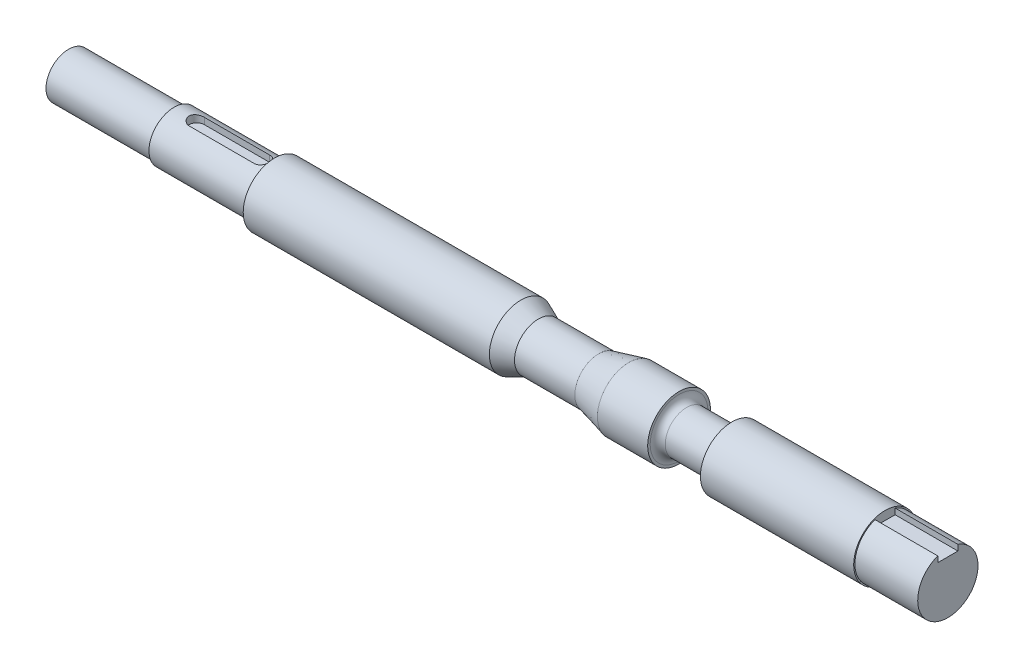
ISO-10303-21;
HEADER;
FILE_DESCRIPTION(('STEP AP214'),'2;1');
FILE_NAME('part.step','',(''),(''),'','','');
FILE_SCHEMA(('AUTOMOTIVE_DESIGN { 1 0 10303 214 1 1 1 1 }'));
ENDSEC;
DATA;
#1=APPLICATION_CONTEXT('core data for automotive mechanical design processes');
#2=APPLICATION_PROTOCOL_DEFINITION('international standard','automotive_design',2000,#1);
#3=PRODUCT_CONTEXT('',#1,'mechanical');
#4=PRODUCT('Part','Part','',(#3));
#5=PRODUCT_RELATED_PRODUCT_CATEGORY('part','',(#4));
#6=PRODUCT_DEFINITION_FORMATION('','',#4);
#7=PRODUCT_DEFINITION_CONTEXT('part definition',#1,'design');
#8=PRODUCT_DEFINITION('design','',#6,#7);
#9=PRODUCT_DEFINITION_SHAPE('','',#8);
#10=(LENGTH_UNIT() NAMED_UNIT(*) SI_UNIT(.MILLI.,.METRE.));
#11=(NAMED_UNIT(*) PLANE_ANGLE_UNIT() SI_UNIT($,.RADIAN.));
#12=(NAMED_UNIT(*) SI_UNIT($,.STERADIAN.) SOLID_ANGLE_UNIT());
#13=UNCERTAINTY_MEASURE_WITH_UNIT(LENGTH_MEASURE(1.E-05),#10,'distance_accuracy_value','');
#14=(GEOMETRIC_REPRESENTATION_CONTEXT(3) GLOBAL_UNCERTAINTY_ASSIGNED_CONTEXT((#13)) GLOBAL_UNIT_ASSIGNED_CONTEXT((#10,
#11,#12)) REPRESENTATION_CONTEXT('',''));
#15=CARTESIAN_POINT('',(0.,0.,0.));
#16=DIRECTION('',(0.,0.,1.));
#17=DIRECTION('',(1.,0.,0.));
#18=AXIS2_PLACEMENT_3D('',#15,#16,#17);
#19=CARTESIAN_POINT('',(0.,9.,0.));
#20=DIRECTION('',(1.,0.,0.));
#21=DIRECTION('',(0.,0.,-1.));
#22=AXIS2_PLACEMENT_3D('',#19,#20,#21);
#23=PLANE('',#22);
#24=CARTESIAN_POINT('',(0.,0.,0.));
#25=DIRECTION('',(-1.,0.,0.));
#26=DIRECTION('',(0.,0.,1.));
#27=AXIS2_PLACEMENT_3D('',#24,#25,#26);
#28=CIRCLE('',#27,9.);
#29=CARTESIAN_POINT('',(0.,0.,9.));
#30=VERTEX_POINT('',#29);
#31=EDGE_CURVE('E158',#30,#30,#28,.T.);
#32=ORIENTED_EDGE('',*,*,#31,.T.);
#33=EDGE_LOOP('',(#32));
#34=FACE_BOUND('',#33,.T.);
#35=ADVANCED_FACE('F39',(#34),#23,.F.);
#36=CARTESIAN_POINT('',(350.,0.,0.));
#37=DIRECTION('',(-1.,0.,0.));
#38=DIRECTION('',(0.,0.,1.));
#39=AXIS2_PLACEMENT_3D('',#36,#37,#38);
#40=PLANE('',#39);
#41=DIRECTION('',(0.,0.,-1.));
#42=VECTOR('',#41,1.);
#43=CARTESIAN_POINT('',(350.,9.,4.));
#44=LINE('',#43,#42);
#45=CARTESIAN_POINT('',(350.,9.,4.));
#46=VERTEX_POINT('',#45);
#47=CARTESIAN_POINT('',(350.,9.,-4.));
#48=VERTEX_POINT('',#47);
#49=EDGE_CURVE('E134',#46,#48,#44,.T.);
#50=ORIENTED_EDGE('',*,*,#49,.F.);
#51=DIRECTION('',(0.,-1.,0.));
#52=VECTOR('',#51,1.);
#53=CARTESIAN_POINT('',(350.,9.,4.));
#54=LINE('',#53,#52);
#55=CARTESIAN_POINT('',(350.,11.3137084989848,4.));
#56=VERTEX_POINT('',#55);
#57=EDGE_CURVE('E138',#56,#46,#54,.T.);
#58=ORIENTED_EDGE('',*,*,#57,.F.);
#59=CARTESIAN_POINT('',(350.,0.,0.));
#60=DIRECTION('',(-1.,0.,0.));
#61=DIRECTION('',(0.,0.,1.));
#62=AXIS2_PLACEMENT_3D('',#59,#60,#61);
#63=CIRCLE('',#62,12.);
#64=CARTESIAN_POINT('',(350.,11.3137084989848,-4.));
#65=VERTEX_POINT('',#64);
#66=EDGE_CURVE('E198',#65,#56,#63,.T.);
#67=ORIENTED_EDGE('',*,*,#66,.F.);
#68=DIRECTION('',(0.,1.,0.));
#69=VECTOR('',#68,1.);
#70=CARTESIAN_POINT('',(350.,9.,-4.));
#71=LINE('',#70,#69);
#72=EDGE_CURVE('E65',#48,#65,#71,.T.);
#73=ORIENTED_EDGE('',*,*,#72,.F.);
#74=EDGE_LOOP('',(#50,#58,#67,#73));
#75=FACE_BOUND('',#74,.T.);
#76=ADVANCED_FACE('F269',(#75),#40,.F.);
#77=CARTESIAN_POINT('',(0.,0.,0.));
#78=DIRECTION('',(-1.,0.,0.));
#79=DIRECTION('',(0.,0.,1.));
#80=AXIS2_PLACEMENT_3D('',#77,#78,#79);
#81=CYLINDRICAL_SURFACE('',#80,12.);
#82=ORIENTED_EDGE('',*,*,#66,.T.);
#83=DIRECTION('',(-1.,0.,0.));
#84=VECTOR('',#83,1.);
#85=CARTESIAN_POINT('',(0.,11.3137084989848,4.));
#86=LINE('',#85,#84);
#87=CARTESIAN_POINT('',(325.,11.3137084989848,4.));
#88=VERTEX_POINT('',#87);
#89=EDGE_CURVE('E156',#56,#88,#86,.T.);
#90=ORIENTED_EDGE('',*,*,#89,.T.);
#91=CARTESIAN_POINT('',(325.,0.,0.));
#92=DIRECTION('',(-1.,0.,0.));
#93=DIRECTION('',(0.,0.,1.));
#94=AXIS2_PLACEMENT_3D('',#91,#92,#93);
#95=CIRCLE('',#94,12.);
#96=CARTESIAN_POINT('',(325.,11.3137084989848,-4.));
#97=VERTEX_POINT('',#96);
#98=EDGE_CURVE('E193',#97,#88,#95,.T.);
#99=ORIENTED_EDGE('',*,*,#98,.F.);
#100=DIRECTION('',(-1.,0.,0.));
#101=VECTOR('',#100,1.);
#102=CARTESIAN_POINT('',(0.,11.3137084989848,-4.));
#103=LINE('',#102,#101);
#104=EDGE_CURVE('E143',#97,#65,#103,.F.);
#105=ORIENTED_EDGE('',*,*,#104,.T.);
#106=EDGE_LOOP('',(#82,#90,#99,#105));
#107=FACE_BOUND('',#106,.T.);
#108=ADVANCED_FACE('F280',(#107),#81,.T.);
#109=CARTESIAN_POINT('',(325.,12.,0.));
#110=DIRECTION('',(-1.,0.,0.));
#111=DIRECTION('',(0.,0.,1.));
#112=AXIS2_PLACEMENT_3D('',#109,#110,#111);
#113=PLANE('',#112);
#114=CARTESIAN_POINT('',(325.,0.,0.));
#115=DIRECTION('',(-1.,0.,0.));
#116=DIRECTION('',(0.,0.,1.));
#117=AXIS2_PLACEMENT_3D('',#114,#115,#116);
#118=CIRCLE('',#117,12.5);
#119=CARTESIAN_POINT('',(325.,0.,12.5));
#120=VERTEX_POINT('',#119);
#121=EDGE_CURVE('E195',#120,#120,#118,.T.);
#122=ORIENTED_EDGE('',*,*,#121,.F.);
#123=EDGE_LOOP('',(#122));
#124=FACE_BOUND('',#123,.T.);
#125=ORIENTED_EDGE('',*,*,#98,.T.);
#126=DIRECTION('',(0.,-1.,0.));
#127=VECTOR('',#126,1.);
#128=CARTESIAN_POINT('',(325.,9.,4.));
#129=LINE('',#128,#127);
#130=CARTESIAN_POINT('',(325.,9.,4.));
#131=VERTEX_POINT('',#130);
#132=EDGE_CURVE('E137',#88,#131,#129,.T.);
#133=ORIENTED_EDGE('',*,*,#132,.T.);
#134=DIRECTION('',(0.,0.,-1.));
#135=VECTOR('',#134,1.);
#136=CARTESIAN_POINT('',(325.,9.,4.));
#137=LINE('',#136,#135);
#138=CARTESIAN_POINT('',(325.,9.,-4.));
#139=VERTEX_POINT('',#138);
#140=EDGE_CURVE('E150',#131,#139,#137,.T.);
#141=ORIENTED_EDGE('',*,*,#140,.T.);
#142=DIRECTION('',(0.,1.,0.));
#143=VECTOR('',#142,1.);
#144=CARTESIAN_POINT('',(325.,9.,-4.));
#145=LINE('',#144,#143);
#146=EDGE_CURVE('E145',#139,#97,#145,.T.);
#147=ORIENTED_EDGE('',*,*,#146,.T.);
#148=EDGE_LOOP('',(#125,#133,#141,#147));
#149=FACE_BOUND('',#148,.T.);
#150=ADVANCED_FACE('F311',(#124,#149),#113,.F.);
#151=CARTESIAN_POINT('',(0.,0.,0.));
#152=DIRECTION('',(-1.,0.,0.));
#153=DIRECTION('',(0.,0.,1.));
#154=AXIS2_PLACEMENT_3D('',#151,#152,#153);
#155=CYLINDRICAL_SURFACE('',#154,12.5);
#156=CARTESIAN_POINT('',(264.,0.,0.));
#157=DIRECTION('',(-1.,0.,0.));
#158=DIRECTION('',(0.,0.,1.));
#159=AXIS2_PLACEMENT_3D('',#156,#157,#158);
#160=CIRCLE('',#159,12.5);
#161=CARTESIAN_POINT('',(264.,0.,12.5));
#162=VERTEX_POINT('',#161);
#163=EDGE_CURVE('E186',#162,#162,#160,.T.);
#164=ORIENTED_EDGE('',*,*,#163,.F.);
#165=EDGE_LOOP('',(#164));
#166=FACE_BOUND('',#165,.T.);
#167=ORIENTED_EDGE('',*,*,#121,.T.);
#168=EDGE_LOOP('',(#167));
#169=FACE_BOUND('',#168,.T.);
#170=ADVANCED_FACE('F302',(#166,#169),#155,.T.);
#171=CARTESIAN_POINT('',(264.,8.5,0.));
#172=DIRECTION('',(1.,0.,0.));
#173=DIRECTION('',(0.,0.,-1.));
#174=AXIS2_PLACEMENT_3D('',#171,#172,#173);
#175=PLANE('',#174);
#176=CARTESIAN_POINT('',(264.,0.,0.));
#177=DIRECTION('',(1.,0.,0.));
#178=DIRECTION('',(0.,0.,-1.));
#179=AXIS2_PLACEMENT_3D('',#176,#177,#178);
#180=CIRCLE('',#179,10.5);
#181=CARTESIAN_POINT('',(264.,0.,-10.5));
#182=VERTEX_POINT('',#181);
#183=EDGE_CURVE('E203',#182,#182,#180,.T.);
#184=ORIENTED_EDGE('',*,*,#183,.T.);
#185=EDGE_LOOP('',(#184));
#186=FACE_BOUND('',#185,.T.);
#187=ORIENTED_EDGE('',*,*,#163,.T.);
#188=EDGE_LOOP('',(#187));
#189=FACE_BOUND('',#188,.T.);
#190=ADVANCED_FACE('F294',(#186,#189),#175,.F.);
#191=CARTESIAN_POINT('',(0.,0.,0.));
#192=DIRECTION('',(-1.,0.,0.));
#193=DIRECTION('',(0.,0.,1.));
#194=AXIS2_PLACEMENT_3D('',#191,#192,#193);
#195=CYLINDRICAL_SURFACE('',#194,8.5);
#196=CARTESIAN_POINT('',(246.,0.,0.));
#197=DIRECTION('',(-1.,0.,0.));
#198=DIRECTION('',(0.,0.,1.));
#199=AXIS2_PLACEMENT_3D('',#196,#197,#198);
#200=CIRCLE('',#199,8.5);
#201=CARTESIAN_POINT('',(246.,0.,8.5));
#202=VERTEX_POINT('',#201);
#203=EDGE_CURVE('E208',#202,#202,#200,.F.);
#204=ORIENTED_EDGE('',*,*,#203,.T.);
#205=EDGE_LOOP('',(#204));
#206=FACE_BOUND('',#205,.T.);
#207=CARTESIAN_POINT('',(262.,0.,0.));
#208=DIRECTION('',(1.,0.,0.));
#209=DIRECTION('',(0.,0.,-1.));
#210=AXIS2_PLACEMENT_3D('',#207,#208,#209);
#211=CIRCLE('',#210,8.5);
#212=CARTESIAN_POINT('',(262.,0.,-8.5));
#213=VERTEX_POINT('',#212);
#214=EDGE_CURVE('E201',#213,#213,#211,.F.);
#215=ORIENTED_EDGE('',*,*,#214,.T.);
#216=EDGE_LOOP('',(#215));
#217=FACE_BOUND('',#216,.T.);
#218=ADVANCED_FACE('F291',(#206,#217),#195,.T.);
#219=CARTESIAN_POINT('',(243.,12.5,0.));
#220=DIRECTION('',(-1.,0.,0.));
#221=DIRECTION('',(0.,0.,1.));
#222=AXIS2_PLACEMENT_3D('',#219,#220,#221);
#223=PLANE('',#222);
#224=CARTESIAN_POINT('',(243.,0.,0.));
#225=DIRECTION('',(-1.,0.,0.));
#226=DIRECTION('',(0.,0.,1.));
#227=AXIS2_PLACEMENT_3D('',#224,#225,#226);
#228=CIRCLE('',#227,11.5);
#229=CARTESIAN_POINT('',(243.,0.,11.5));
#230=VERTEX_POINT('',#229);
#231=EDGE_CURVE('E210',#230,#230,#228,.T.);
#232=ORIENTED_EDGE('',*,*,#231,.T.);
#233=EDGE_LOOP('',(#232));
#234=FACE_BOUND('',#233,.T.);
#235=CARTESIAN_POINT('',(243.,0.,0.));
#236=DIRECTION('',(-1.,0.,0.));
#237=DIRECTION('',(0.,0.,1.));
#238=AXIS2_PLACEMENT_3D('',#235,#236,#237);
#239=CIRCLE('',#238,12.5);
#240=CARTESIAN_POINT('',(243.,0.,12.5));
#241=VERTEX_POINT('',#240);
#242=EDGE_CURVE('E187',#241,#241,#239,.T.);
#243=ORIENTED_EDGE('',*,*,#242,.F.);
#244=EDGE_LOOP('',(#243));
#245=FACE_BOUND('',#244,.T.);
#246=ADVANCED_FACE('F295',(#234,#245),#223,.F.);
#247=CARTESIAN_POINT('',(0.,0.,0.));
#248=DIRECTION('',(-1.,0.,0.));
#249=DIRECTION('',(0.,0.,1.));
#250=AXIS2_PLACEMENT_3D('',#247,#248,#249);
#251=CYLINDRICAL_SURFACE('',#250,12.5);
#252=CARTESIAN_POINT('',(223.,0.,0.));
#253=DIRECTION('',(-1.,0.,0.));
#254=DIRECTION('',(0.,0.,1.));
#255=AXIS2_PLACEMENT_3D('',#252,#253,#254);
#256=CIRCLE('',#255,12.5);
#257=CARTESIAN_POINT('',(223.,0.,12.5));
#258=VERTEX_POINT('',#257);
#259=EDGE_CURVE('E182',#258,#258,#256,.T.);
#260=ORIENTED_EDGE('',*,*,#259,.F.);
#261=EDGE_LOOP('',(#260));
#262=FACE_BOUND('',#261,.T.);
#263=ORIENTED_EDGE('',*,*,#242,.T.);
#264=EDGE_LOOP('',(#263));
#265=FACE_BOUND('',#264,.T.);
#266=ADVANCED_FACE('F301',(#262,#265),#251,.T.);
#267=CARTESIAN_POINT('',(223.,0.,0.));
#268=DIRECTION('',(1.,0.,0.));
#269=DIRECTION('',(0.,0.,-1.));
#270=AXIS2_PLACEMENT_3D('',#267,#268,#269);
#271=CONICAL_SURFACE('',#270,12.5,0.244978663126863);
#272=CARTESIAN_POINT('',(211.,0.,0.));
#273=DIRECTION('',(-1.,0.,0.));
#274=DIRECTION('',(0.,0.,1.));
#275=AXIS2_PLACEMENT_3D('',#272,#273,#274);
#276=CIRCLE('',#275,9.5);
#277=CARTESIAN_POINT('',(211.,0.,9.5));
#278=VERTEX_POINT('',#277);
#279=EDGE_CURVE('E179',#278,#278,#276,.T.);
#280=ORIENTED_EDGE('',*,*,#279,.F.);
#281=EDGE_LOOP('',(#280));
#282=FACE_BOUND('',#281,.T.);
#283=ORIENTED_EDGE('',*,*,#259,.T.);
#284=EDGE_LOOP('',(#283));
#285=FACE_BOUND('',#284,.T.);
#286=ADVANCED_FACE('F449',(#282,#285),#271,.T.);
#287=CARTESIAN_POINT('',(0.,0.,0.));
#288=DIRECTION('',(-1.,0.,0.));
#289=DIRECTION('',(0.,0.,1.));
#290=AXIS2_PLACEMENT_3D('',#287,#288,#289);
#291=CYLINDRICAL_SURFACE('',#290,9.5);
#292=CARTESIAN_POINT('',(187.,0.,0.));
#293=DIRECTION('',(-1.,0.,0.));
#294=DIRECTION('',(0.,0.,1.));
#295=AXIS2_PLACEMENT_3D('',#292,#293,#294);
#296=CIRCLE('',#295,9.5);
#297=CARTESIAN_POINT('',(187.,0.,9.5));
#298=VERTEX_POINT('',#297);
#299=EDGE_CURVE('E180',#298,#298,#296,.T.);
#300=ORIENTED_EDGE('',*,*,#299,.F.);
#301=EDGE_LOOP('',(#300));
#302=FACE_BOUND('',#301,.T.);
#303=ORIENTED_EDGE('',*,*,#279,.T.);
#304=EDGE_LOOP('',(#303));
#305=FACE_BOUND('',#304,.T.);
#306=ADVANCED_FACE('F437',(#302,#305),#291,.T.);
#307=CARTESIAN_POINT('',(187.,0.,0.));
#308=DIRECTION('',(-1.,0.,0.));
#309=DIRECTION('',(0.,0.,1.));
#310=AXIS2_PLACEMENT_3D('',#307,#308,#309);
#311=CONICAL_SURFACE('',#310,9.5,0.404891786285081);
#312=CARTESIAN_POINT('',(180.,0.,0.));
#313=DIRECTION('',(-1.,0.,0.));
#314=DIRECTION('',(0.,0.,1.));
#315=AXIS2_PLACEMENT_3D('',#312,#313,#314);
#316=CIRCLE('',#315,12.5);
#317=CARTESIAN_POINT('',(180.,0.,12.5));
#318=VERTEX_POINT('',#317);
#319=EDGE_CURVE('E172',#318,#318,#316,.T.);
#320=ORIENTED_EDGE('',*,*,#319,.F.);
#321=EDGE_LOOP('',(#320));
#322=FACE_BOUND('',#321,.T.);
#323=ORIENTED_EDGE('',*,*,#299,.T.);
#324=EDGE_LOOP('',(#323));
#325=FACE_BOUND('',#324,.T.);
#326=ADVANCED_FACE('F427',(#322,#325),#311,.T.);
#327=CARTESIAN_POINT('',(0.,0.,0.));
#328=DIRECTION('',(-1.,0.,0.));
#329=DIRECTION('',(0.,0.,1.));
#330=AXIS2_PLACEMENT_3D('',#327,#328,#329);
#331=CYLINDRICAL_SURFACE('',#330,12.5);
#332=CARTESIAN_POINT('',(82.,0.,0.));
#333=DIRECTION('',(-1.,0.,0.));
#334=DIRECTION('',(0.,0.,1.));
#335=AXIS2_PLACEMENT_3D('',#332,#333,#334);
#336=CIRCLE('',#335,12.5);
#337=CARTESIAN_POINT('',(82.,0.,12.5));
#338=VERTEX_POINT('',#337);
#339=EDGE_CURVE('E171',#338,#338,#336,.T.);
#340=ORIENTED_EDGE('',*,*,#339,.F.);
#341=EDGE_LOOP('',(#340));
#342=FACE_BOUND('',#341,.T.);
#343=ORIENTED_EDGE('',*,*,#319,.T.);
#344=EDGE_LOOP('',(#343));
#345=FACE_BOUND('',#344,.T.);
#346=ADVANCED_FACE('F422',(#342,#345),#331,.T.);
#347=CARTESIAN_POINT('',(82.,12.5,0.));
#348=DIRECTION('',(1.,0.,0.));
#349=DIRECTION('',(0.,0.,-1.));
#350=AXIS2_PLACEMENT_3D('',#347,#348,#349);
#351=PLANE('',#350);
#352=CARTESIAN_POINT('',(82.,0.,0.));
#353=DIRECTION('',(-1.,0.,0.));
#354=DIRECTION('',(0.,0.,1.));
#355=AXIS2_PLACEMENT_3D('',#352,#353,#354);
#356=CIRCLE('',#355,10.);
#357=CARTESIAN_POINT('',(82.,0.,10.));
#358=VERTEX_POINT('',#357);
#359=EDGE_CURVE('E166',#358,#358,#356,.T.);
#360=ORIENTED_EDGE('',*,*,#359,.F.);
#361=EDGE_LOOP('',(#360));
#362=FACE_BOUND('',#361,.T.);
#363=ORIENTED_EDGE('',*,*,#339,.T.);
#364=EDGE_LOOP('',(#363));
#365=FACE_BOUND('',#364,.T.);
#366=ADVANCED_FACE('F264',(#362,#365),#351,.F.);
#367=CARTESIAN_POINT('',(0.,0.,0.));
#368=DIRECTION('',(-1.,0.,0.));
#369=DIRECTION('',(0.,0.,1.));
#370=AXIS2_PLACEMENT_3D('',#367,#368,#369);
#371=CYLINDRICAL_SURFACE('',#370,10.);
#372=DIRECTION('',(-1.,0.,0.));
#373=VECTOR('',#372,1.);
#374=CARTESIAN_POINT('',(0.,9.53939201416945,-3.));
#375=LINE('',#374,#373);
#376=CARTESIAN_POINT('',(51.,9.53939201416945,-3.));
#377=VERTEX_POINT('',#376);
#378=CARTESIAN_POINT('',(77.,9.53939201416945,-3.));
#379=VERTEX_POINT('',#378);
#380=EDGE_CURVE('E11',#377,#379,#375,.F.);
#381=ORIENTED_EDGE('',*,*,#380,.T.);
#382=CARTESIAN_POINT('',(77.,9.53939201416945,-3.));
#383=CARTESIAN_POINT('',(77.0823355208227,9.53938054248206,-3.00001027845728));
#384=CARTESIAN_POINT('',(77.1646644550632,9.54045772064378,-2.99661062684472));
#385=CARTESIAN_POINT('',(77.3286939527654,9.54470412105986,-2.98307142899347));
#386=CARTESIAN_POINT('',(77.4103946533244,9.54787287296848,-2.97293339805418));
#387=CARTESIAN_POINT('',(77.5723849156732,9.55620668351003,-2.94603140625045));
#388=CARTESIAN_POINT('',(77.652677524043,9.56136667250114,-2.92928426957737));
#389=CARTESIAN_POINT('',(77.8114758441342,9.57351626651178,-2.88932853030395));
#390=CARTESIAN_POINT('',(77.8899815090674,9.58050591937827,-2.86611975872641));
#391=CARTESIAN_POINT('',(78.1219493879901,9.60391637654136,-2.78708584446024));
#392=CARTESIAN_POINT('',(78.272068438833,9.6227900783039,-2.72181852542973));
#393=CARTESIAN_POINT('',(78.559226043979,9.66493213967819,-2.56815043531276));
#394=CARTESIAN_POINT('',(78.6962584707622,9.6882025429064,-2.4797388992416));
#395=CARTESIAN_POINT('',(78.9577229879478,9.73733650515374,-2.27929879634443));
#396=CARTESIAN_POINT('',(79.0816848740609,9.76325505469873,-2.16666914746584));
#397=CARTESIAN_POINT('',(79.3092736148387,9.81429628475077,-1.92227736150433));
#398=CARTESIAN_POINT('',(79.412897033861,9.8394188301941,-1.79051199848164));
#399=CARTESIAN_POINT('',(79.5989268650946,9.88666477976534,-1.50821997465697));
#400=CARTESIAN_POINT('',(79.6808501797826,9.90871541546877,-1.35736167401016));
#401=CARTESIAN_POINT('',(79.8179770040029,9.94668940088144,-1.04324233568302));
#402=CARTESIAN_POINT('',(79.873187403368,9.96261433032402,-0.879984508687979));
#403=CARTESIAN_POINT('',(79.953759551791,9.98615279768397,-0.550649404820596));
#404=CARTESIAN_POINT('',(79.9799297035176,9.99399098526792,-0.384786253016199));
#405=CARTESIAN_POINT('',(80.004234695146,10.0012640407204,-0.0508471415689249));
#406=CARTESIAN_POINT('',(80.0023748426782,10.0007004995012,0.117228393125341));
#407=CARTESIAN_POINT('',(79.9712141793085,9.99139205125586,0.445143199271825));
#408=CARTESIAN_POINT('',(79.9427893091919,9.98290831016512,0.605074290763028));
#409=CARTESIAN_POINT('',(79.8607367303745,9.95903027401822,0.917780104370313));
#410=CARTESIAN_POINT('',(79.8071077013173,9.94363561692558,1.07055445110879));
#411=CARTESIAN_POINT('',(79.6755755564752,9.90730429851782,1.36669563173912));
#412=CARTESIAN_POINT('',(79.5973967112239,9.88630511384914,1.50993201207613));
#413=CARTESIAN_POINT('',(79.4192028199656,9.84099249303646,1.78153105916101));
#414=CARTESIAN_POINT('',(79.3191828810593,9.81667831471806,1.90989038323251));
#415=CARTESIAN_POINT('',(79.0956160238154,9.7662334714278,2.15330901082205));
#416=CARTESIAN_POINT('',(78.9713122724738,9.74006890899097,2.26766702955975));
#417=CARTESIAN_POINT('',(78.7050051531489,9.68968430229327,2.47413538985067));
#418=CARTESIAN_POINT('',(78.5629966392702,9.66546482675133,2.5662392402618));
#419=CARTESIAN_POINT('',(78.2634381431001,9.62154457591303,2.72632814481701));
#420=CARTESIAN_POINT('',(78.1057456408129,9.60189192491895,2.79406012682263));
#421=CARTESIAN_POINT('',(77.7805509920369,9.56991327306402,2.90171772009405));
#422=CARTESIAN_POINT('',(77.6130642785713,9.55757606951749,2.94168586436072));
#423=CARTESIAN_POINT('',(77.3700102218596,9.54628064650011,2.97802407180159));
#424=CARTESIAN_POINT('',(77.2962185316408,9.54370312550533,2.98626405978017));
#425=CARTESIAN_POINT('',(77.1482970418009,9.54025857223564,2.99724711229708));
#426=CARTESIAN_POINT('',(77.0741679006723,9.53938902493288,2.99999825936538));
#427=CARTESIAN_POINT('',(77.,9.53939201416945,3.));
#428=B_SPLINE_CURVE_WITH_KNOTS('',3,(#382,#383,#384,#385,#386,#387,#388,#389,#390,#391,#392,
#393,#394,#395,#396,#397,#398,#399,#400,#401,#402,#403,#404,#405,#406,#407,#408,#409,#410,#411,
#412,#413,#414,#415,#416,#417,#418,#419,#420,#421,#422,#423,#424,#425,#426,#427),.UNSPECIFIED.,
.F.,.F.,(4,2,2,2,2,2,2,2,2,2,2,2,2,2,2,2,2,2,2,2,2,2,4),(0.,0.246918142439488,0.493780777706094,
0.740019009623012,0.986263681482027,1.47813347402025,1.97023245590778,2.47635119822767,
2.98255536239033,3.49922810620071,4.01576751791673,4.51753600864765,5.01920948804101,
5.50490358251093,5.99062312360832,6.48200583350622,6.97349873739171,7.48389234847123,
7.99443465298716,8.51013494368214,9.02504345105574,9.24774267716778,9.47011372732391),.UNSPECIFIED.);
#429=CARTESIAN_POINT('',(77.,9.53939201416945,3.));
#430=VERTEX_POINT('',#429);
#431=EDGE_CURVE('E214',#379,#430,#428,.T.);
#432=ORIENTED_EDGE('',*,*,#431,.T.);
#433=DIRECTION('',(-1.,0.,0.));
#434=VECTOR('',#433,1.);
#435=CARTESIAN_POINT('',(0.,9.53939201416945,3.));
#436=LINE('',#435,#434);
#437=CARTESIAN_POINT('',(51.,9.53939201416945,3.));
#438=VERTEX_POINT('',#437);
#439=EDGE_CURVE('E50',#430,#438,#436,.T.);
#440=ORIENTED_EDGE('',*,*,#439,.T.);
#441=CARTESIAN_POINT('',(51.,9.53939201416945,3.));
#442=CARTESIAN_POINT('',(50.9176644791773,9.53938054248206,3.00001027845728));
#443=CARTESIAN_POINT('',(50.8353355449368,9.54045772064378,2.99661062684472));
#444=CARTESIAN_POINT('',(50.6713060472345,9.54470412105986,2.98307142899347));
#445=CARTESIAN_POINT('',(50.5896053466756,9.54787287296848,2.97293339805418));
#446=CARTESIAN_POINT('',(50.4276150843268,9.55620668351003,2.94603140625045));
#447=CARTESIAN_POINT('',(50.347322475957,9.56136667250114,2.92928426957737));
#448=CARTESIAN_POINT('',(50.1885241558658,9.57351626651178,2.88932853030395));
#449=CARTESIAN_POINT('',(50.1100184909326,9.58050591937827,2.8661197587264));
#450=CARTESIAN_POINT('',(49.8780506120098,9.60391637654136,2.78708584446024));
#451=CARTESIAN_POINT('',(49.727931561167,9.62279007830391,2.72181852542972));
#452=CARTESIAN_POINT('',(49.4407739560209,9.66493213967819,2.56815043531276));
#453=CARTESIAN_POINT('',(49.3037415292378,9.68820254290641,2.4797388992416));
#454=CARTESIAN_POINT('',(49.0422770120522,9.73733650515374,2.27929879634442));
#455=CARTESIAN_POINT('',(48.9183151259391,9.76325505469874,2.16666914746584));
#456=CARTESIAN_POINT('',(48.6907263851612,9.81429628475077,1.92227736150433));
#457=CARTESIAN_POINT('',(48.587102966139,9.8394188301941,1.79051199848164));
#458=CARTESIAN_POINT('',(48.4010731349054,9.88666477976534,1.50821997465697));
#459=CARTESIAN_POINT('',(48.3191498202174,9.90871541546877,1.35736167401016));
#460=CARTESIAN_POINT('',(48.1820229959971,9.94668940088144,1.04324233568303));
#461=CARTESIAN_POINT('',(48.126812596632,9.96261433032402,0.879984508687983));
#462=CARTESIAN_POINT('',(48.046240448209,9.98615279768397,0.550649404820599));
#463=CARTESIAN_POINT('',(48.0200702964824,9.99399098526792,0.384786253016201));
#464=CARTESIAN_POINT('',(47.9957653048539,10.0012640407204,0.0508471415689268));
#465=CARTESIAN_POINT('',(47.9976251573218,10.0007004995012,-0.11722839312534));
#466=CARTESIAN_POINT('',(48.0287858206914,9.99139205125586,-0.445143199271826));
#467=CARTESIAN_POINT('',(48.0572106908081,9.98290831016512,-0.60507429076303));
#468=CARTESIAN_POINT('',(48.1392632696255,9.95903027401822,-0.917780104370317));
#469=CARTESIAN_POINT('',(48.1928922986827,9.94363561692558,-1.07055445110879));
#470=CARTESIAN_POINT('',(48.3244244435247,9.90730429851782,-1.36669563173912));
#471=CARTESIAN_POINT('',(48.4026032887761,9.88630511384914,-1.50993201207613));
#472=CARTESIAN_POINT('',(48.5807971800344,9.84099249303646,-1.781531059161));
#473=CARTESIAN_POINT('',(48.6808171189407,9.81667831471806,-1.90989038323251));
#474=CARTESIAN_POINT('',(48.9043839761846,9.7662334714278,-2.15330901082206));
#475=CARTESIAN_POINT('',(49.0286877275262,9.74006890899097,-2.26766702955976));
#476=CARTESIAN_POINT('',(49.2949948468511,9.68968430229327,-2.47413538985067));
#477=CARTESIAN_POINT('',(49.4370033607298,9.66546482675133,-2.5662392402618));
#478=CARTESIAN_POINT('',(49.7365618568999,9.62154457591303,-2.72632814481702));
#479=CARTESIAN_POINT('',(49.8942543591871,9.60189192491895,-2.79406012682263));
#480=CARTESIAN_POINT('',(50.2194490079631,9.56991327306402,-2.90171772009405));
#481=CARTESIAN_POINT('',(50.3869357214287,9.55757606951749,-2.94168586436072));
#482=CARTESIAN_POINT('',(50.6299897781404,9.54628064650011,-2.97802407180159));
#483=CARTESIAN_POINT('',(50.7037814683592,9.54370312550533,-2.98626405978017));
#484=CARTESIAN_POINT('',(50.851702958199,9.54025857223564,-2.99724711229709));
#485=CARTESIAN_POINT('',(50.9258320993277,9.53938902493288,-2.99999825936538));
#486=CARTESIAN_POINT('',(51.,9.53939201416945,-3.));
#487=B_SPLINE_CURVE_WITH_KNOTS('',3,(#441,#442,#443,#444,#445,#446,#447,#448,#449,#450,#451,
#452,#453,#454,#455,#456,#457,#458,#459,#460,#461,#462,#463,#464,#465,#466,#467,#468,#469,#470,
#471,#472,#473,#474,#475,#476,#477,#478,#479,#480,#481,#482,#483,#484,#485,#486),.UNSPECIFIED.,
.F.,.F.,(4,2,2,2,2,2,2,2,2,2,2,2,2,2,2,2,2,2,2,2,2,2,4),(0.,0.246918142439467,0.493780777706094,
0.74001900962302,0.986263681482027,1.47813347402026,1.97023245590779,2.47635119822766,
2.98255536239032,3.4992281062007,4.01576751791672,4.51753600864764,5.01920948804101,
5.50490358251093,5.99062312360832,6.48200583350621,6.9734987373917,7.48389234847122,
7.99443465298715,8.51013494368215,9.02504345105574,9.24774267716779,9.47011372732391),.UNSPECIFIED.);
#488=EDGE_CURVE('E53',#438,#377,#487,.T.);
#489=ORIENTED_EDGE('',*,*,#488,.T.);
#490=EDGE_LOOP('',(#381,#432,#440,#489));
#491=FACE_BOUND('',#490,.T.);
#492=CARTESIAN_POINT('',(42.,0.,0.));
#493=DIRECTION('',(-1.,0.,0.));
#494=DIRECTION('',(0.,0.,1.));
#495=AXIS2_PLACEMENT_3D('',#492,#493,#494);
#496=CIRCLE('',#495,10.);
#497=CARTESIAN_POINT('',(42.,0.,10.));
#498=VERTEX_POINT('',#497);
#499=EDGE_CURVE('E164',#498,#498,#496,.T.);
#500=ORIENTED_EDGE('',*,*,#499,.F.);
#501=EDGE_LOOP('',(#500));
#502=FACE_BOUND('',#501,.T.);
#503=ORIENTED_EDGE('',*,*,#359,.T.);
#504=EDGE_LOOP('',(#503));
#505=FACE_BOUND('',#504,.T.);
#506=ADVANCED_FACE('F227',(#491,#502,#505),#371,.T.);
#507=CARTESIAN_POINT('',(42.,10.,0.));
#508=DIRECTION('',(1.,0.,0.));
#509=DIRECTION('',(0.,0.,-1.));
#510=AXIS2_PLACEMENT_3D('',#507,#508,#509);
#511=PLANE('',#510);
#512=CARTESIAN_POINT('',(42.,0.,0.));
#513=DIRECTION('',(-1.,0.,0.));
#514=DIRECTION('',(0.,0.,1.));
#515=AXIS2_PLACEMENT_3D('',#512,#513,#514);
#516=CIRCLE('',#515,9.);
#517=CARTESIAN_POINT('',(42.,0.,9.));
#518=VERTEX_POINT('',#517);
#519=EDGE_CURVE('E162',#518,#518,#516,.T.);
#520=ORIENTED_EDGE('',*,*,#519,.F.);
#521=EDGE_LOOP('',(#520));
#522=FACE_BOUND('',#521,.T.);
#523=ORIENTED_EDGE('',*,*,#499,.T.);
#524=EDGE_LOOP('',(#523));
#525=FACE_BOUND('',#524,.T.);
#526=ADVANCED_FACE('F260',(#522,#525),#511,.F.);
#527=CARTESIAN_POINT('',(0.,0.,0.));
#528=DIRECTION('',(-1.,0.,0.));
#529=DIRECTION('',(0.,0.,1.));
#530=AXIS2_PLACEMENT_3D('',#527,#528,#529);
#531=CYLINDRICAL_SURFACE('',#530,9.);
#532=ORIENTED_EDGE('',*,*,#31,.F.);
#533=EDGE_LOOP('',(#532));
#534=FACE_BOUND('',#533,.T.);
#535=ORIENTED_EDGE('',*,*,#519,.T.);
#536=EDGE_LOOP('',(#535));
#537=FACE_BOUND('',#536,.T.);
#538=ADVANCED_FACE('F251',(#534,#537),#531,.T.);
#539=CARTESIAN_POINT('',(262.,0.,0.));
#540=DIRECTION('',(1.,0.,0.));
#541=DIRECTION('',(0.,0.,-1.));
#542=AXIS2_PLACEMENT_3D('',#539,#540,#541);
#543=TOROIDAL_SURFACE('',#542,10.5,2.);
#544=ORIENTED_EDGE('',*,*,#183,.F.);
#545=EDGE_LOOP('',(#544));
#546=FACE_BOUND('',#545,.T.);
#547=ORIENTED_EDGE('',*,*,#214,.F.);
#548=EDGE_LOOP('',(#547));
#549=FACE_BOUND('',#548,.T.);
#550=ADVANCED_FACE('F257',(#546,#549),#543,.F.);
#551=CARTESIAN_POINT('',(246.,0.,0.));
#552=DIRECTION('',(-1.,0.,0.));
#553=DIRECTION('',(0.,0.,1.));
#554=AXIS2_PLACEMENT_3D('',#551,#552,#553);
#555=TOROIDAL_SURFACE('',#554,11.5,3.);
#556=ORIENTED_EDGE('',*,*,#203,.F.);
#557=EDGE_LOOP('',(#556));
#558=FACE_BOUND('',#557,.T.);
#559=ORIENTED_EDGE('',*,*,#231,.F.);
#560=EDGE_LOOP('',(#559));
#561=FACE_BOUND('',#560,.T.);
#562=ADVANCED_FACE('F41',(#558,#561),#555,.F.);
#563=CARTESIAN_POINT('',(315.,9.,4.));
#564=DIRECTION('',(0.,0.,1.));
#565=DIRECTION('',(0.,-1.,0.));
#566=AXIS2_PLACEMENT_3D('',#563,#564,#565);
#567=PLANE('',#566);
#568=ORIENTED_EDGE('',*,*,#57,.T.);
#569=DIRECTION('',(1.,0.,0.));
#570=VECTOR('',#569,1.);
#571=CARTESIAN_POINT('',(315.,9.,4.));
#572=LINE('',#571,#570);
#573=EDGE_CURVE('E148',#131,#46,#572,.T.);
#574=ORIENTED_EDGE('',*,*,#573,.F.);
#575=ORIENTED_EDGE('',*,*,#132,.F.);
#576=ORIENTED_EDGE('',*,*,#89,.F.);
#577=EDGE_LOOP('',(#568,#574,#575,#576));
#578=FACE_BOUND('',#577,.T.);
#579=ADVANCED_FACE('F250',(#578),#567,.F.);
#580=CARTESIAN_POINT('',(315.,9.,-4.));
#581=DIRECTION('',(0.,0.,-1.));
#582=DIRECTION('',(-1.,0.,0.));
#583=AXIS2_PLACEMENT_3D('',#580,#581,#582);
#584=PLANE('',#583);
#585=ORIENTED_EDGE('',*,*,#146,.F.);
#586=DIRECTION('',(1.,0.,0.));
#587=VECTOR('',#586,1.);
#588=CARTESIAN_POINT('',(315.,9.,-4.));
#589=LINE('',#588,#587);
#590=EDGE_CURVE('E147',#139,#48,#589,.T.);
#591=ORIENTED_EDGE('',*,*,#590,.T.);
#592=ORIENTED_EDGE('',*,*,#72,.T.);
#593=ORIENTED_EDGE('',*,*,#104,.F.);
#594=EDGE_LOOP('',(#585,#591,#592,#593));
#595=FACE_BOUND('',#594,.T.);
#596=ADVANCED_FACE('F242',(#595),#584,.F.);
#597=CARTESIAN_POINT('',(315.,9.,4.));
#598=DIRECTION('',(0.,-1.,0.));
#599=DIRECTION('',(0.,0.,-1.));
#600=AXIS2_PLACEMENT_3D('',#597,#598,#599);
#601=PLANE('',#600);
#602=ORIENTED_EDGE('',*,*,#573,.T.);
#603=ORIENTED_EDGE('',*,*,#49,.T.);
#604=ORIENTED_EDGE('',*,*,#590,.F.);
#605=ORIENTED_EDGE('',*,*,#140,.F.);
#606=EDGE_LOOP('',(#602,#603,#604,#605));
#607=FACE_BOUND('',#606,.T.);
#608=ADVANCED_FACE('F243',(#607),#601,.F.);
#609=CARTESIAN_POINT('',(51.,7.,0.));
#610=DIRECTION('',(0.,1.,0.));
#611=DIRECTION('',(0.,0.,1.));
#612=AXIS2_PLACEMENT_3D('',#609,#610,#611);
#613=CYLINDRICAL_SURFACE('',#612,3.);
#614=DIRECTION('',(0.,1.,0.));
#615=VECTOR('',#614,1.);
#616=CARTESIAN_POINT('',(51.,7.,3.));
#617=LINE('',#616,#615);
#618=CARTESIAN_POINT('',(51.,7.,3.));
#619=VERTEX_POINT('',#618);
#620=EDGE_CURVE('E101',#619,#438,#617,.T.);
#621=ORIENTED_EDGE('',*,*,#620,.F.);
#622=CARTESIAN_POINT('',(51.,7.,0.));
#623=DIRECTION('',(0.,1.,0.));
#624=DIRECTION('',(0.,0.,1.));
#625=AXIS2_PLACEMENT_3D('',#622,#623,#624);
#626=CIRCLE('',#625,3.);
#627=CARTESIAN_POINT('',(51.,7.,-3.));
#628=VERTEX_POINT('',#627);
#629=EDGE_CURVE('E110',#628,#619,#626,.T.);
#630=ORIENTED_EDGE('',*,*,#629,.F.);
#631=DIRECTION('',(0.,1.,0.));
#632=VECTOR('',#631,1.);
#633=CARTESIAN_POINT('',(51.,7.,-3.));
#634=LINE('',#633,#632);
#635=EDGE_CURVE('E126',#628,#377,#634,.T.);
#636=ORIENTED_EDGE('',*,*,#635,.T.);
#637=ORIENTED_EDGE('',*,*,#488,.F.);
#638=EDGE_LOOP('',(#621,#630,#636,#637));
#639=FACE_BOUND('',#638,.T.);
#640=ADVANCED_FACE('F102',(#639),#613,.F.);
#641=CARTESIAN_POINT('',(51.,7.,-3.));
#642=DIRECTION('',(0.,0.,-1.));
#643=DIRECTION('',(-1.,0.,0.));
#644=AXIS2_PLACEMENT_3D('',#641,#642,#643);
#645=PLANE('',#644);
#646=ORIENTED_EDGE('',*,*,#635,.F.);
#647=DIRECTION('',(-1.,0.,0.));
#648=VECTOR('',#647,1.);
#649=CARTESIAN_POINT('',(51.,7.,-3.));
#650=LINE('',#649,#648);
#651=CARTESIAN_POINT('',(77.,7.,-3.));
#652=VERTEX_POINT('',#651);
#653=EDGE_CURVE('E115',#652,#628,#650,.T.);
#654=ORIENTED_EDGE('',*,*,#653,.F.);
#655=DIRECTION('',(0.,1.,0.));
#656=VECTOR('',#655,1.);
#657=CARTESIAN_POINT('',(77.,7.,-3.));
#658=LINE('',#657,#656);
#659=EDGE_CURVE('E131',#652,#379,#658,.T.);
#660=ORIENTED_EDGE('',*,*,#659,.T.);
#661=ORIENTED_EDGE('',*,*,#380,.F.);
#662=EDGE_LOOP('',(#646,#654,#660,#661));
#663=FACE_BOUND('',#662,.T.);
#664=ADVANCED_FACE('F236',(#663),#645,.F.);
#665=CARTESIAN_POINT('',(77.,7.,0.));
#666=DIRECTION('',(0.,1.,0.));
#667=DIRECTION('',(0.,0.,1.));
#668=AXIS2_PLACEMENT_3D('',#665,#666,#667);
#669=CYLINDRICAL_SURFACE('',#668,3.);
#670=ORIENTED_EDGE('',*,*,#659,.F.);
#671=CARTESIAN_POINT('',(77.,7.,0.));
#672=DIRECTION('',(0.,1.,0.));
#673=DIRECTION('',(0.,0.,1.));
#674=AXIS2_PLACEMENT_3D('',#671,#672,#673);
#675=CIRCLE('',#674,3.);
#676=CARTESIAN_POINT('',(77.,7.,3.));
#677=VERTEX_POINT('',#676);
#678=EDGE_CURVE('E122',#677,#652,#675,.T.);
#679=ORIENTED_EDGE('',*,*,#678,.F.);
#680=DIRECTION('',(0.,1.,0.));
#681=VECTOR('',#680,1.);
#682=CARTESIAN_POINT('',(77.,7.,3.));
#683=LINE('',#682,#681);
#684=EDGE_CURVE('E111',#677,#430,#683,.T.);
#685=ORIENTED_EDGE('',*,*,#684,.T.);
#686=ORIENTED_EDGE('',*,*,#431,.F.);
#687=EDGE_LOOP('',(#670,#679,#685,#686));
#688=FACE_BOUND('',#687,.T.);
#689=ADVANCED_FACE('F233',(#688),#669,.F.);
#690=CARTESIAN_POINT('',(51.,7.,3.));
#691=DIRECTION('',(0.,0.,1.));
#692=DIRECTION('',(1.,0.,0.));
#693=AXIS2_PLACEMENT_3D('',#690,#691,#692);
#694=PLANE('',#693);
#695=ORIENTED_EDGE('',*,*,#684,.F.);
#696=DIRECTION('',(1.,0.,0.));
#697=VECTOR('',#696,1.);
#698=CARTESIAN_POINT('',(51.,7.,3.));
#699=LINE('',#698,#697);
#700=EDGE_CURVE('E114',#619,#677,#699,.T.);
#701=ORIENTED_EDGE('',*,*,#700,.F.);
#702=ORIENTED_EDGE('',*,*,#620,.T.);
#703=ORIENTED_EDGE('',*,*,#439,.F.);
#704=EDGE_LOOP('',(#695,#701,#702,#703));
#705=FACE_BOUND('',#704,.T.);
#706=ADVANCED_FACE('F116',(#705),#694,.F.);
#707=CARTESIAN_POINT('',(51.,7.,0.));
#708=DIRECTION('',(0.,1.,0.));
#709=DIRECTION('',(0.,0.,1.));
#710=AXIS2_PLACEMENT_3D('',#707,#708,#709);
#711=PLANE('',#710);
#712=ORIENTED_EDGE('',*,*,#629,.T.);
#713=ORIENTED_EDGE('',*,*,#700,.T.);
#714=ORIENTED_EDGE('',*,*,#678,.T.);
#715=ORIENTED_EDGE('',*,*,#653,.T.);
#716=EDGE_LOOP('',(#712,#713,#714,#715));
#717=FACE_BOUND('',#716,.T.);
#718=ADVANCED_FACE('F124',(#717),#711,.T.);
#719=CLOSED_SHELL('',(#35,#76,#108,#150,#170,#190,#218,#246,#266,#286,#306,#326,#346,#366,#506,
#526,#538,#550,#562,#579,#596,#608,#640,#664,#689,#706,#718));
#720=MANIFOLD_SOLID_BREP('B2',#719);
#721=ADVANCED_BREP_SHAPE_REPRESENTATION('',(#18,#720),#14);
#722=SHAPE_DEFINITION_REPRESENTATION(#9,#721);
ENDSEC;
END-ISO-10303-21;
